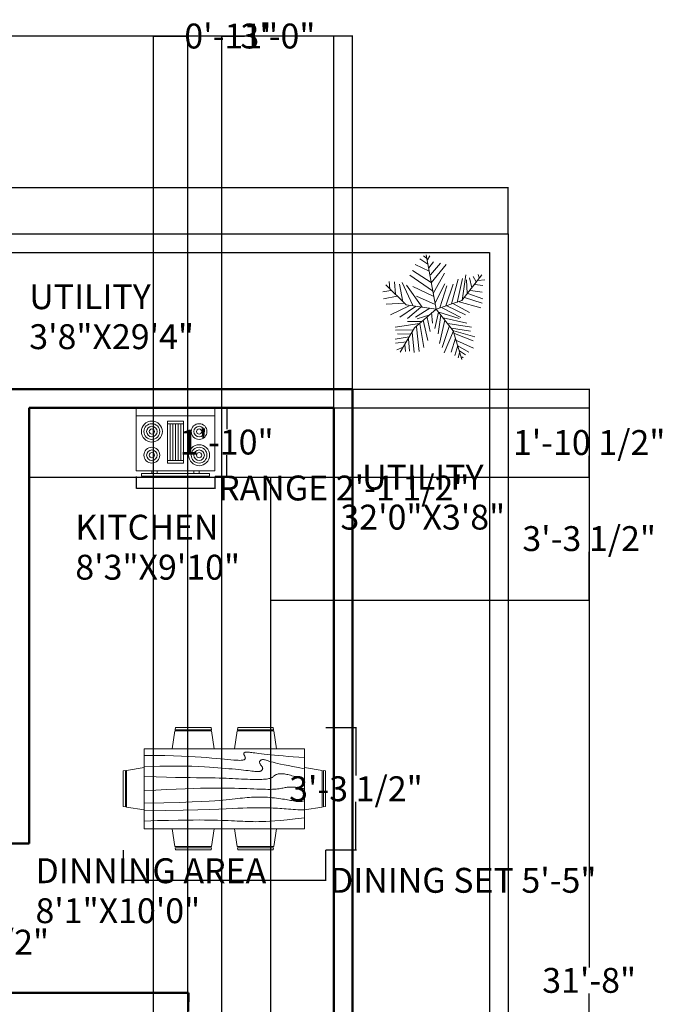
# Model space of a CAD drawing. Units: inches. Extents: x -1912 to -1462, y -785 to -198.
# Tile 3 of 3: x -1668 to -1462, y -515 to -198. Entities that reach past the tile are written whole.
import ezdxf
from ezdxf.enums import TextEntityAlignment as Align

# ---------------------------------------------------------------- set-up
doc = ezdxf.new("R2010")
doc.units = ezdxf.units.IN
doc.header["$MEASUREMENT"] = 0
for name, color, linetype, lineweight in [('A-ANNO-DIMS', 2, 'Continuous', 18), ('A-AREA-IDEN', 7, 'Continuous', 18), ('A-EQPM', 9, 'Continuous', 18), ('A-FLOR-CASE', 9, 'Continuous', 25), ('A-FURN', 8, 'Continuous', 18), ('A-WALL', 7, 'Continuous', 50), ('C-PROP', 8, 'Continuous', 25), ('L-PLNT-TREE', 3, 'Continuous', 13)]:
    doc.layers.add(name, color=color, linetype=linetype, lineweight=lineweight)
doc.styles.get("Standard").update_dxf_attribs({"font": 'arial.ttf'})
doc.dimstyles.get("Standard").update_dxf_attribs({"dimtxt": 8, "dimasz": 0.18, "dimexe": 0.18, "dimexo": 0.0625, "dimgap": 0.09, "dimtad": 0, "dimtih": 1, "dimtoh": 1, "dimzin": 0, "dimdsep": 46, "dimlunit": 3, "dimtxsty": 'Standard', "dimcen": 0.09, "dimadec": 0, "dimazin": 0, "dimtfac": 1, "dimtofl": 0, "dimtmove": 0, "dimatfit": 3, "dimfxl": 1, "dimtolj": 1, "dimtzin": 0, "dimarcsym": 0})

# ---------------------------------------------------------------- blocks, each defined once
blk = doc.blocks.new('Dining Set - 36 x 72 in.')
for p, q in [((-22, 27.5), (-22.1562, 26.50042)), ((-22, 27.5), (-6, 27.5)), ((-5.8437, 26.49966), (-6, 27.5)), ((6, 27.5), (5.8438, 26.50042)), ((6, 27.5), (22, 27.5)), ((22.1563, 26.49966), (22, 27.5)), ((-22.2343, 26.00059), (-23.4847, 17.99762)), ((-22.2304, 26), (-5.7608, 26)), ((-5.8416, 26.5), (-22.1534, 26.5)), ((-4.5152, 17.99762), (-5.7655, 25.99926)), ((5.7657, 26.00059), (4.5153, 17.99762)), ((5.7696, 26), (22.2392, 26)), ((22.1584, 26.5), (5.8466, 26.5)), ((23.4848, 17.99762), (22.2345, 25.99926)), ((36, 18), (-36, 18)), ((-36, 18), (-36, -18)), ((36, -18), (36, 18)), ((-44.0006, 8.23428), (-35.9976, 9.48474)), ((44.0006, 8.23428), (35.9976, 9.48474)), ((-45.5, 8), (-44.5004, 8.15617)), ((-45.5, 8), (-45.5, -8)), ((-44.5, -8.15843), (-44.5, 8.15338)), ((-44, 8.23041), (-44, -8.23915)), ((44, 8.23041), (44, -8.23915)), ((44.5, -8.15843), (44.5, 8.15338)), ((45.5, 8), (44.5005, 8.15617)), ((45.5, 8), (45.5, -8)), ((-44.4997, -8.15631), (-45.5, -8)), ((-35.9976, -9.48476), (-43.9993, -8.2345)), ((35.9976, -9.48476), (43.9993, -8.2345)), ((44.4997, -8.15631), (45.5, -8)), ((-36, -18), (36, -18)), ((-22.2343, -26.0006), (-23.4847, -17.99762)), ((-4.5152, -17.99762), (-5.7655, -25.99928)), ((5.7657, -26.0006), (4.5153, -17.99762)), ((23.4848, -17.99762), (22.2345, -25.99928)), ((-22.2304, -26), (-5.7608, -26)), ((-22, -27.5), (-22.1562, -26.50044)), ((-5.8416, -26.5), (-22.1534, -26.5)), ((-5.8437, -26.49967), (-6, -27.5)), ((5.7696, -26), (22.2392, -26)), ((6, -27.5), (5.8438, -26.50044)), ((22.1584, -26.5), (5.8466, -26.5)), ((22.1563, -26.49967), (22, -27.5)), ((-22, -27.5), (-6, -27.5)), ((6, -27.5), (22, -27.5))]:
    blk.add_line(p, q)
for points in [[(-36, 15), (-31.1772, 14.97754), (-26.8079, 14.91406), (-22.8538, 14.81543), (-19.276, 14.6875), (-16.0362, 14.53613), (-13.0957, 14.36718), (-10.4159, 14.18652), (-7.9583, 14), (-5.6904, 13.81315), (-3.6035, 13.63021), (-1.6954, 13.45508), (0.0365, 13.29166), (1.5945, 13.14388), (2.9811, 13.01562), (4.1988, 12.9108), (5.25, 12.83333), (6.1393, 12.78613), (6.8802, 12.76823), (7.4883, 12.77767), (7.9792, 12.8125), (8.3685, 12.87077), (8.6719, 12.95052), (8.9049, 13.0498), (9.0833, 13.16666), (9.2205, 13.29899), (9.3216, 13.44401), (9.3895, 13.59879), (9.4271, 13.76041), (9.4373, 13.92594), (9.4232, 14.09245), (9.3875, 14.257), (9.3333, 14.41666), (9.2638, 14.56917), (9.1836, 14.71484), (9.0975, 14.85465), (9.0104, 14.98958), (8.9272, 15.1206), (8.8529, 15.2487), (8.7922, 15.37483), (8.75, 15.5), (8.7305, 15.62467), (8.7344, 15.74739), (8.7617, 15.86621), (8.8125, 15.97916), (8.8867, 16.08431), (8.9844, 16.17968), (9.1055, 16.26334), (9.25, 16.33333), (9.4189, 16.38802), (9.6172, 16.42708), (9.8506, 16.45052), (10.125, 16.45833), (10.4463, 16.45052), (10.8203, 16.42708), (11.2529, 16.38802), (11.75, 16.33333), (12.3184, 16.26318), (12.9694, 16.17838), (13.7151, 16.07991), (14.5677, 15.96875), (15.5395, 15.84586), (16.6426, 15.71224), (17.8893, 15.56884), (19.2917, 15.41666), (20.859, 15.25667), (22.5879, 15.08984), (24.4721, 14.91715), (26.5052, 14.73958), (28.6809, 14.5581), (30.9929, 14.3737), (33.4347, 14.18733), (36, 14)], [(-36, 10), (-28.9766, 10.14274), (-23.1725, 10.20442), (-18.4241, 10.19775), (-14.5677, 10.13541), (-11.4399, 10.03011), (-8.877, 9.89453), (-6.7154, 9.74137), (-4.7917, 9.58333), (-2.9698, 9.43082), (-1.2246, 9.28515), (0.4415, 9.14534), (2.026, 9.01041), (3.5266, 8.87939), (4.9408, 8.7513), (6.266, 8.62516), (7.5, 8.5), (8.6411, 8.37549), (9.6914, 8.2539), (10.6538, 8.13818), (11.5312, 8.03125), (12.3267, 7.93603), (13.043, 7.85547), (13.6831, 7.79248), (14.25, 7.75), (14.7471, 7.7303), (15.1797, 7.73307), (15.5537, 7.75732), (15.875, 7.80208), (16.1494, 7.86637), (16.3828, 7.94922), (16.5811, 8.04964), (16.75, 8.16666), (16.8944, 8.29915), (17.0143, 8.44531), (17.1089, 8.60319), (17.1771, 8.77083), (17.218, 8.94629), (17.2305, 9.1276), (17.2137, 9.31282), (17.1667, 9.5), (17.0895, 9.6875), (16.987, 9.875), (16.8649, 10.0625), (16.7292, 10.25), (16.5856, 10.4375), (16.4401, 10.625), (16.2985, 10.8125), (16.1667, 11), (16.05, 11.18733), (15.9518, 11.3737), (15.8752, 11.5581), (15.8229, 11.73958), (15.798, 11.91715), (15.8034, 12.08984), (15.842, 12.25667), (15.9167, 12.41666), (16.0295, 12.56836), (16.1784, 12.70833), (16.3605, 12.83268), (16.5729, 12.9375), (16.8127, 13.01888), (17.0768, 13.07291), (17.3625, 13.0957), (17.6667, 13.08333), (17.9894, 13.03312), (18.3418, 12.94726), (18.7382, 12.82918), (19.1927, 12.68229), (19.7195, 12.51001), (20.3327, 12.31575), (21.0465, 12.10294), (21.875, 11.875), (22.8357, 11.63354), (23.959, 11.37304), (25.2786, 11.08618), (26.8282, 10.76562), (28.6414, 10.40405), (30.752, 9.99414), (33.1936, 9.52856), (36, 9)], [(-36, 5.5), (-30.7157, 5.3348), (-26.069, 5.20963), (-21.9946, 5.11767), (-18.4271, 5.05208), (-15.3009, 5.00602), (-12.5508, 4.97265), (-10.1112, 4.94515), (-7.9167, 4.91666), (-5.909, 4.88167), (-4.0586, 4.83984), (-2.3429, 4.79215), (-0.7396, 4.73958), (0.7739, 4.6831), (2.22, 4.6237), (3.6213, 4.56233), (5, 4.5), (6.373, 4.43782), (7.7344, 4.3776), (9.0723, 4.32129), (10.375, 4.27083), (11.6309, 4.22819), (12.8281, 4.19531), (13.9551, 4.17415), (15, 4.16666), (15.954, 4.17448), (16.819, 4.19791), (17.6001, 4.23698), (18.3021, 4.29166), (18.9299, 4.36198), (19.4883, 4.44791), (19.9823, 4.54948), (20.4167, 4.66666), (20.7969, 4.79899), (21.1302, 4.94401), (21.4245, 5.09879), (21.6875, 5.26041), (21.9271, 5.42594), (22.1511, 5.59245), (22.3672, 5.757), (22.5834, 5.91666), (22.8065, 6.06868), (23.0404, 6.21093), (23.2879, 6.34147), (23.5521, 6.45833), (23.8358, 6.55957), (24.142, 6.64323), (24.4735, 6.70735), (24.8334, 6.75), (25.2235, 6.76969), (25.642, 6.76692), (26.0858, 6.74267), (26.5521, 6.69791), (27.0379, 6.63362), (27.5404, 6.55078), (28.0565, 6.45036), (28.5834, 6.33333), (29.1242, 6.19987), (29.7071, 6.04687), (30.3661, 5.87044), (31.1354, 5.66666), (32.0493, 5.43164), (33.142, 5.16146), (34.4475, 4.85221), (36, 4.5)], [(-36, -1), (-30.7915, -0.6591), (-26.0195, -0.38216), (-21.6519, -0.16284), (-17.6563, 0.00521), (-14.0005, 0.12833), (-10.6523, 0.21289), (-7.5796, 0.26522), (-4.75, 0.29166), (-2.134, 0.29793), (0.2878, 0.28711), (2.5317, 0.26163), (4.6146, 0.22396), (6.5529, 0.17651), (8.3633, 0.12174), (10.0623, 0.06209), (11.6667, 0), (13.1899, -0.06201), (14.6341, -0.1211), (15.9982, -0.17432), (17.2813, -0.21875), (18.4823, -0.25147), (19.6003, -0.26953), (20.6343, -0.27002), (21.5834, -0.25), (22.4481, -0.20768), (23.2357, -0.14584), (23.9549, -0.06836), (24.6146, 0.02083), (25.2235, 0.11784), (25.7904, 0.21875), (26.3241, 0.31966), (26.8334, 0.41666), (27.3265, 0.50618), (27.8099, 0.58593), (28.2894, 0.65397), (28.7709, 0.70833), (29.2601, 0.74707), (29.763, 0.76823), (30.2855, 0.76985), (30.8334, 0.75), (31.4088, 0.70784), (31.9994, 0.64713), (32.589, 0.57275), (33.1615, 0.48958), (33.7008, 0.4025), (34.1908, 0.3164), (34.6153, 0.23616), (34.9584, 0.16666), (35.2099, 0.11165), (35.3848, 0.07031), (35.504, 0.04069), (35.5886, 0.02083), (35.6594, 0.00879), (35.7377, 0.0026), (35.8442, 0.00032), (36, 0)], [(-36, -6.5), (-27.1843, -6.31267), (-20.084, -6.1263), (-14.469, -5.9419), (-10.1094, -5.76042), (-6.7752, -5.58285), (-4.2363, -5.41016), (-2.2629, -5.24333), (-0.625, -5.08334), (0.8708, -4.93099), (2.2715, -4.78646), (3.5872, -4.64974), (4.8281, -4.52084), (6.0046, -4.39974), (7.127, -4.28646), (8.2053, -4.18099), (9.25, -4.08334), (10.2705, -3.99382), (11.2734, -3.91407), (12.2647, -3.84603), (13.25, -3.79167), (14.2354, -3.75293), (15.2266, -3.73177), (16.2295, -3.73015), (17.25, -3.75), (18.2912, -3.79248), (19.3451, -3.85547), (20.4009, -3.93604), (21.4479, -4.03125), (22.4754, -4.13819), (23.4727, -4.25391), (24.4289, -4.37549), (25.3334, -4.5), (26.1785, -4.62492), (26.9694, -4.74935), (27.7145, -4.87281), (28.4219, -4.99479), (29.1, -5.11483), (29.7572, -5.23242), (30.4016, -5.34709), (31.0417, -5.45834), (31.6837, -5.56437), (32.3262, -5.65821), (32.9658, -5.73153), (33.599, -5.77604), (34.2224, -5.78345), (34.8327, -5.74545), (35.4264, -5.65373), (36, -5.5)], [(-36, -10), (-26.4022, -9.81299), (-18.4675, -9.62891), (-11.9839, -9.45069), (-6.7396, -9.28125), (-2.5226, -9.12354), (0.8789, -8.98047), (3.6769, -8.85498), (6.0833, -8.75), (8.2767, -8.66765), (10.3021, -8.60677), (12.1712, -8.56543), (13.8958, -8.54167), (15.4876, -8.53353), (16.9583, -8.53907), (18.3197, -8.55632), (19.5834, -8.58334), (20.7616, -8.61841), (21.8685, -8.66081), (22.9188, -8.71004), (23.9271, -8.76563), (24.9081, -8.82707), (25.8763, -8.89388), (26.8465, -8.96558), (27.8334, -9.04167), (28.8474, -9.12118), (29.8828, -9.20117), (30.93, -9.27824), (31.9792, -9.34896), (33.0205, -9.40991), (34.0443, -9.45768), (35.0407, -9.48885), (36, -9.5)], [(-36, -14.5), (-30.0881, -14.33513), (-25.0332, -14.21224), (-20.7312, -14.12647), (-17.0781, -14.07292), (-13.97, -14.04671), (-11.3027, -14.04297), (-8.9724, -14.05681), (-6.875, -14.08334), (-4.9224, -14.11833), (-3.0905, -14.16016), (-1.3709, -14.20785), (0.2448, -14.26042), (1.7647, -14.3169), (3.1973, -14.3763), (4.5507, -14.43767), (5.8333, -14.5), (7.0554, -14.5621), (8.235, -14.62175), (9.3922, -14.67652), (10.5469, -14.72396), (11.7192, -14.76164), (12.929, -14.78711), (14.1965, -14.79794), (15.5417, -14.79167), (16.9933, -14.76424), (18.6152, -14.70508), (20.4804, -14.60197), (22.6615, -14.44271), (25.2312, -14.21509), (28.2624, -13.9069), (31.8277, -13.50594), (36, -13)]]:
    blk.add_lwpolyline(points)
blk = doc.blocks.new('Range-Oven - 30 in top')
for p, q in [((0, -3), (30, -3)), ((12, -6), (18, -6)), ((13, -20), (13, -6)), ((14, -6), (14, -20)), ((15, -20), (15, -6)), ((16, -6), (16, -20)), ((17, -20), (17, -6)), ((18, -20), (12, -20)), ((6, -24), (6, -25)), ((8, -25), (8, -24)), ((22, -25), (22, -24)), ((24, -24), (24, -25))]:
    blk.add_line(p, q)
for points in [[(0, -24), (0, 0), (30, 0), (30, -24)], [(12, -21), (12, -5), (18, -5), (18, -21)], [(2, -26), (2, -25), (28, -25), (28, -26)]]:
    blk.add_lwpolyline(points, close=True)
for centre, radius in [((6, -9), 4), ((6, -9), 3), ((6, -9), 2), ((24, -9), 3), ((24, -9), 2), ((6, -9), 1), ((24, -9), 1), ((24, -18), 4), ((6, -18), 3), ((6, -18), 2), ((6, -18), 1), ((24, -18), 3), ((24, -18), 2), ((24, -18), 1)]:
    blk.add_circle(centre, radius)
blk = doc.blocks.new('*U11')
for p, q in [((-8.737, 47.138), (-17.069, 52.711)), ((-10.186, 53.64), (-13.084, 55.962)), ((0, 0), (-10.5, 57)), ((-9.099, 51.782), (-6.563, 55.962)), ((-7.288, 39.707), (-21.778, 46.673)), ((-7.65, 43.423), (-2.578, 49.46)), ((-5.839, 35.992), (4.667, 48.067)), ((-5.114, 27.632), (10.463, 46.673)), ((-3.665, 19.273), (-27.574, 35.527)), ((-5.114, 28.097), (-24.676, 40.636)), ((-2.941, 16.486), (8.652, 37.85)), ((16.259, 5.805), (23.142, 31.348)), ((22.055, 7.198), (27.489, 32.277)), ((27, 9), (48, 36)), ((27.127, 9.056), (31.112, 35.992)), ((35.096, 32.741), (37.27, 22.524)), ((38.719, 34.134), (41.979, 28.561)), ((44.153, 36.456), (45.239, 32.741)), ((-31.5, 4.5), (-52.5, 25.5)), ((-48.585, 21.131), (-49.309, 29.026)), ((-43.513, 28.561), (-42.427, 15.558)), ((-38.442, 26.239), (-34.819, 7.663)), ((-35.544, 28.097), (-24.314, 3.947)), ((-14.533, 2.09), (-30.834, 25.31)), ((-24.314, 23.917), (-2.941, 13.7)), ((-1.129, 6.734), (9.014, 26.704)), ((3.942, 1.625), (11.187, 24.381)), ((10.101, 3.483), (17.708, 26.239)), ((31.836, 30.883), (32.561, 16.486)), ((40.53, 25.775), (48.862, 24.846)), ((43.791, 29.954), (51.036, 30.883)), ((-47.498, 19.737), (-55.83, 18.344)), ((-40.615, 13.7), (-55.105, 10.913)), ((-20.691, 13.7), (-1.129, 4.876)), ((29.662, 12.307), (48.137, 6.269)), ((33.285, 16.486), (48.862, 10.913)), ((36.183, 19.737), (48.137, 17.88)), ((-33.37, 6.269), (-52.207, 5.34)), ((-28.299, 3.483), (-47.86, -5.805)), ((-21.416, 3.018), (-38.079, -8.128)), ((0, 0), (-31.5, 4.5)), ((-15.982, 2.09), (-30.11, -9.521)), ((0, 0), (-22.5, -19.5)), ((-6.563, 1.161), (-21.416, -8.128)), ((0, 0), (27, 9)), ((0, 0), (18, -22.5)), ((6.478, 1.625), (26.04, -8.592)), ((11.187, 3.483), (30.749, -5.805)), ((18.07, 5.805), (35.096, -3.483)), ((24.229, 7.663), (46.688, 1.625)), ((-6.563, -5.805), (-19.967, -9.985)), ((-9.461, -8.592), (-6.201, -23.453)), ((-4.752, -3.483), (-3.665, -14.629)), ((2.493, -3.019), (-1.491, -20.202)), ((1.769, -2.555), (24.229, -9.521)), ((5.029, -6.27), (2.131, -25.775)), ((7.565, -9.056), (32.198, -14.629)), ((-17.431, -15.094), (-42.789, -18.809)), ((-22.5, -19.5), (-37.5, -45)), ((-15.257, -12.772), (-30.11, -12.772)), ((-20.691, -18.345), (-17.793, -44.352)), ((-17.069, -15.094), (-12.721, -40.172)), ((-13.446, -11.378), (-8.737, -32.741)), ((9.014, -11.378), (3.58, -35.992)), ((14.085, -16.951), (6.478, -40.172)), ((12.274, -15.094), (36.907, -18.809)), ((16.259, -19.738), (36.183, -22.989)), ((-28.299, -29.026), (-42.789, -31.348)), ((-24.314, -21.596), (-42.427, -22.06)), ((-26.849, -26.24), (-40.253, -25.775)), ((-29.023, -30.884), (-27.936, -43.887)), ((-25.038, -23.918), (-22.865, -45.281)), ((18.07, -22.524), (8.289, -45.745)), ((20.244, -30.419), (15.897, -44.816)), ((18, -22.5), (27, -52.5)), ((18.433, -22.524), (40.53, -29.026)), ((19.157, -25.311), (38.719, -33.206)), ((-30.834, -34.135), (-42.427, -35.528)), ((-34.457, -39.708), (-40.978, -42.494)), ((-32.646, -36.921), (-31.921, -44.352)), ((22.78, -37.85), (19.519, -48.532)), ((21.331, -32.741), (39.081, -40.636)), ((22.78, -38.314), (34.372, -44.816)), ((24.591, -45.745), (23.142, -50.854)), ((24.591, -43.423), (30.749, -47.603)), ((26.764, -49.925), (28.213, -50.854))]:
    blk.add_line(p, q)
blk = doc.blocks.new('*D12')
at = {"layer": 'A-ANNO-DIMS', "color": 0, "lineweight": -2, "transparency": 16777216}
for p, q in [((-1871.08, -267.18), (-1871.08, -252.32)), ((-1870.9, -252.5), (-1697.95, -252.5)), ((-1511.26, -252.5), (-1684.2, -252.5)), ((-1511.08, -267.18), (-1511.08, -252.32))]:
    blk.add_line(p, q, dxfattribs=at)
at = {"layer": 'A-ANNO-DIMS', "color": 0, "transparency": 16777216}
for points in [[(-1870.9, -252.47), (-1870.9, -252.53), (-1871.08, -252.5)], [(-1511.26, -252.47), (-1511.26, -252.53), (-1511.08, -252.5)]]:
    blk.add_solid(points, dxfattribs=at)
at = {"layer": 'Defpoints', "color": 0, "transparency": 16777216}
for p in [(-1511.08, -252.5), (-1871.08, -267.24), (-1511.08, -267.24)]:
    blk.add_point(p, dxfattribs=at)
at = {"layer": 'A-ANNO-DIMS', "color": 0, "transparency": 16777216, "insert": (-1691.08, -252.5), "char_height": 8, "attachment_point": 5}
blk.add_mtext("\\A1;30'", dxfattribs=at)
blk = doc.blocks.new('*D17')
at = {"layer": 'A-ANNO-DIMS', "color": 0, "lineweight": -2, "transparency": 16777216}
for p, q in [((-1742.16, -491.83), (-1742.16, -495.14)), ((-1720.86, -491.83), (-1720.86, -495.14)), ((-1741.98, -494.96), (-1721.04, -494.96)), ((-1720.86, -494.96), (-1720.68, -494.96))]:
    blk.add_line(p, q, dxfattribs=at)
at = {"layer": 'A-ANNO-DIMS', "color": 0, "transparency": 16777216}
for points in [[(-1741.98, -494.93), (-1741.98, -494.99), (-1742.16, -494.96)], [(-1721.04, -494.93), (-1721.04, -494.99), (-1720.86, -494.96)]]:
    blk.add_solid(points, dxfattribs=at)
at = {"layer": 'Defpoints', "color": 0, "transparency": 16777216}
for p in [(-1742.16, -491.77), (-1720.86, -491.77), (-1720.86, -494.96)]:
    blk.add_point(p, dxfattribs=at)
at = {"layer": 'A-ANNO-DIMS', "color": 0, "transparency": 16777216, "insert": (-1689.61, -494.96), "char_height": 8, "attachment_point": 5}
blk.add_mtext('\\A1;WC 1\'-9 1/2"', dxfattribs=at)
blk = doc.blocks.new('*D27')
at = {"layer": 'A-ANNO-DIMS', "color": 0, "lineweight": -2, "transparency": 16777216}
for p, q in [((-1634.83, -465.38), (-1634.83, -475.26)), ((-1569.75, -465.38), (-1569.75, -475.26)), ((-1634.65, -475.08), (-1569.93, -475.08)), ((-1569.75, -475.08), (-1569.57, -475.08))]:
    blk.add_line(p, q, dxfattribs=at)
at = {"layer": 'A-ANNO-DIMS', "color": 0, "transparency": 16777216}
for points in [[(-1634.65, -475.05), (-1634.65, -475.11), (-1634.83, -475.08)], [(-1569.93, -475.05), (-1569.93, -475.11), (-1569.75, -475.08)]]:
    blk.add_solid(points, dxfattribs=at)
at = {"layer": 'Defpoints', "color": 0, "transparency": 16777216}
for p in [(-1634.83, -465.31), (-1569.75, -465.31), (-1569.75, -475.08)]:
    blk.add_point(p, dxfattribs=at)
at = {"layer": 'A-ANNO-DIMS', "color": 0, "transparency": 16777216, "insert": (-1525.52, -475.08), "char_height": 8, "attachment_point": 5}
blk.add_mtext('\\A1;DINING SET 5\'-5"', dxfattribs=at)
blk = doc.blocks.new('*D28')
at = {"layer": 'A-ANNO-DIMS', "color": 0, "lineweight": -2, "transparency": 16777216}
for p, q in [((-1569.69, -425.98), (-1559.81, -425.98)), ((-1559.99, -426.16), (-1559.99, -441.42)), ((-1559.99, -465.13), (-1559.99, -449.88)), ((-1569.69, -465.31), (-1559.81, -465.31))]:
    blk.add_line(p, q, dxfattribs=at)
at = {"layer": 'A-ANNO-DIMS', "color": 0, "transparency": 16777216}
for points in [[(-1560.02, -426.16), (-1559.96, -426.16), (-1559.99, -425.98)], [(-1560.02, -465.13), (-1559.96, -465.13), (-1559.99, -465.31)]]:
    blk.add_solid(points, dxfattribs=at)
at = {"layer": 'Defpoints', "color": 0, "transparency": 16777216}
for p in [(-1569.75, -425.98), (-1559.99, -425.98), (-1569.75, -465.31)]:
    blk.add_point(p, dxfattribs=at)
at = {"layer": 'A-ANNO-DIMS', "color": 0, "transparency": 16777216, "insert": (-1559.99, -445.65), "char_height": 8, "attachment_point": 5}
blk.add_mtext('\\A1;3\'-3 1/2"', dxfattribs=at)
blk = doc.blocks.new('*D31')
at = {"layer": 'A-ANNO-DIMS', "color": 0, "lineweight": -2, "transparency": 16777216}
for p, q in [((-1630.66, -345.25), (-1630.66, -349.17)), ((-1605.34, -345.25), (-1605.34, -349.17)), ((-1630.48, -348.99), (-1605.52, -348.99)), ((-1605.34, -348.99), (-1605.16, -348.99))]:
    blk.add_line(p, q, dxfattribs=at)
at = {"layer": 'A-ANNO-DIMS', "color": 0, "transparency": 16777216}
for points in [[(-1630.48, -348.96), (-1630.48, -349.02), (-1630.66, -348.99)], [(-1605.52, -348.96), (-1605.52, -349.02), (-1605.34, -348.99)]]:
    blk.add_solid(points, dxfattribs=at)
at = {"layer": 'Defpoints', "color": 0, "transparency": 16777216}
for p in [(-1630.66, -345.19), (-1605.34, -345.19), (-1605.34, -348.99)]:
    blk.add_point(p, dxfattribs=at)
at = {"layer": 'A-ANNO-DIMS', "color": 0, "transparency": 16777216, "insert": (-1563.9, -348.99), "char_height": 8, "attachment_point": 5}
blk.add_mtext('\\A1;RANGE 2\'-1 1/2"', dxfattribs=at)
blk = doc.blocks.new('*D32')
at = {"layer": 'A-ANNO-DIMS', "color": 0, "lineweight": -2, "transparency": 16777216}
for p, q in [((-1605.28, -323.25), (-1601.36, -323.25)), ((-1601.54, -323.43), (-1601.54, -330.04)), ((-1601.54, -345.01), (-1601.54, -338.39)), ((-1605.28, -345.19), (-1601.36, -345.19))]:
    blk.add_line(p, q, dxfattribs=at)
at = {"layer": 'A-ANNO-DIMS', "color": 0, "transparency": 16777216}
for points in [[(-1601.57, -323.43), (-1601.51, -323.43), (-1601.54, -323.25)], [(-1601.57, -345.01), (-1601.51, -345.01), (-1601.54, -345.19)]]:
    blk.add_solid(points, dxfattribs=at)
at = {"layer": 'Defpoints', "color": 0, "transparency": 16777216}
for p in [(-1605.34, -323.25), (-1601.54, -323.25), (-1605.34, -345.19)]:
    blk.add_point(p, dxfattribs=at)
at = {"layer": 'A-ANNO-DIMS', "color": 0, "transparency": 16777216, "insert": (-1601.54, -334.22), "char_height": 8, "attachment_point": 5}
blk.add_mtext('\\A1;1\'-10"', dxfattribs=at)
blk = doc.blocks.new('*D33')
at = {"layer": 'A-ANNO-DIMS', "color": 0, "lineweight": -2, "transparency": 16777216}
for p, q in [((-1821.08, -317.18), (-1821.08, -203.54)), ((-1820.9, -203.72), (-1704.98, -203.72)), ((-1561.26, -203.72), (-1677.18, -203.72)), ((-1561.08, -317.18), (-1561.08, -203.54))]:
    blk.add_line(p, q, dxfattribs=at)
at = {"layer": 'A-ANNO-DIMS', "color": 0, "transparency": 16777216}
for points in [[(-1820.9, -203.69), (-1820.9, -203.75), (-1821.08, -203.72)], [(-1561.26, -203.69), (-1561.26, -203.75), (-1561.08, -203.72)]]:
    blk.add_solid(points, dxfattribs=at)
at = {"layer": 'Defpoints', "color": 0, "transparency": 16777216}
for p in [(-1561.08, -203.72), (-1821.08, -317.24), (-1561.08, -317.24)]:
    blk.add_point(p, dxfattribs=at)
at = {"layer": 'A-ANNO-DIMS', "color": 0, "transparency": 16777216, "insert": (-1691.08, -203.72), "char_height": 8, "attachment_point": 5}
blk.add_mtext('\\A1;21\'-8"', dxfattribs=at)
blk = doc.blocks.new('*D34')
at = {"layer": 'A-ANNO-DIMS', "color": 0, "lineweight": -2, "transparency": 16777216}
for p, q in [((-1561.02, -317.24), (-1484.85, -317.24)), ((-1485.03, -317.42), (-1485.03, -503.06)), ((-1485.03, -697.06), (-1485.03, -511.42)), ((-1561.02, -697.24), (-1484.85, -697.24))]:
    blk.add_line(p, q, dxfattribs=at)
at = {"layer": 'A-ANNO-DIMS', "color": 0, "transparency": 16777216}
for points in [[(-1485.06, -317.42), (-1485, -317.42), (-1485.03, -317.24)], [(-1485.06, -697.06), (-1485, -697.06), (-1485.03, -697.24)]]:
    blk.add_solid(points, dxfattribs=at)
at = {"layer": 'Defpoints', "color": 0, "transparency": 16777216}
for p in [(-1561.08, -317.24), (-1561.08, -697.24), (-1485.03, -697.24)]:
    blk.add_point(p, dxfattribs=at)
at = {"layer": 'A-ANNO-DIMS', "color": 0, "transparency": 16777216, "insert": (-1485.03, -507.24), "char_height": 8, "attachment_point": 5}
blk.add_mtext('\\A1;31\'-8"', dxfattribs=at)
blk = doc.blocks.new('*D38')
at = {"layer": 'A-ANNO-DIMS', "color": 0, "lineweight": -2, "transparency": 16777216}
for p, q in [((-1603.08, -578.18), (-1603.08, -203.54)), ((-1602.9, -203.72), (-1595.8, -203.72)), ((-1567.26, -203.72), (-1574.36, -203.72)), ((-1567.08, -578.18), (-1567.08, -203.54))]:
    blk.add_line(p, q, dxfattribs=at)
at = {"layer": 'A-ANNO-DIMS', "color": 0, "transparency": 16777216}
for points in [[(-1602.9, -203.69), (-1602.9, -203.75), (-1603.08, -203.72)], [(-1567.26, -203.69), (-1567.26, -203.75), (-1567.08, -203.72)]]:
    blk.add_solid(points, dxfattribs=at)
at = {"layer": 'Defpoints', "color": 0, "transparency": 16777216}
for p in [(-1567.08, -203.72), (-1603.08, -578.24), (-1567.08, -578.24)]:
    blk.add_point(p, dxfattribs=at)
at = {"layer": 'A-ANNO-DIMS', "color": 0, "transparency": 16777216, "insert": (-1585.08, -203.72), "char_height": 8, "attachment_point": 5}
blk.add_mtext('\\A1;3\'-0"', dxfattribs=at)
blk = doc.blocks.new('*D39')
at = {"layer": 'A-ANNO-DIMS', "color": 0, "lineweight": -2, "transparency": 16777216}
for p, q in [((-1625.08, -655.18), (-1625.08, -203.54)), ((-1624.9, -203.72), (-1614.26, -203.72)), ((-1614.08, -655.18), (-1614.08, -203.54)), ((-1614.08, -203.72), (-1613.9, -203.72))]:
    blk.add_line(p, q, dxfattribs=at)
at = {"layer": 'A-ANNO-DIMS', "color": 0, "transparency": 16777216}
for points in [[(-1624.9, -203.69), (-1624.9, -203.75), (-1625.08, -203.72)], [(-1614.26, -203.69), (-1614.26, -203.75), (-1614.08, -203.72)]]:
    blk.add_solid(points, dxfattribs=at)
at = {"layer": 'Defpoints', "color": 0, "transparency": 16777216}
for p in [(-1614.08, -203.72), (-1625.08, -655.24), (-1614.08, -655.24)]:
    blk.add_point(p, dxfattribs=at)
at = {"layer": 'A-ANNO-DIMS', "color": 0, "transparency": 16777216, "insert": (-1600.07, -203.72), "char_height": 8, "attachment_point": 5}
blk.add_mtext('\\A1;0\'-11"', dxfattribs=at)
blk = doc.blocks.new('*D41')
at = {"layer": 'A-ANNO-DIMS', "color": 0, "lineweight": -2, "transparency": 16777216}
for p, q in [((-1665.02, -323.24), (-1484.85, -323.24)), ((-1485.03, -323.42), (-1485.03, -330.14)), ((-1485.03, -345.32), (-1485.03, -338.6)), ((-1665.02, -345.5), (-1484.85, -345.5))]:
    blk.add_line(p, q, dxfattribs=at)
at = {"layer": 'A-ANNO-DIMS', "color": 0, "transparency": 16777216}
for points in [[(-1485.06, -323.42), (-1485, -323.42), (-1485.03, -323.24)], [(-1485.06, -345.32), (-1485, -345.32), (-1485.03, -345.5)]]:
    blk.add_solid(points, dxfattribs=at)
at = {"layer": 'Defpoints', "color": 0, "transparency": 16777216}
for p in [(-1665.08, -323.24), (-1665.08, -345.5), (-1485.03, -345.5)]:
    blk.add_point(p, dxfattribs=at)
at = {"layer": 'A-ANNO-DIMS', "color": 0, "transparency": 16777216, "insert": (-1485.03, -334.37), "char_height": 8, "attachment_point": 5}
blk.add_mtext('\\A1;1\'-10 1/2"', dxfattribs=at)
blk = doc.blocks.new('*D42')
at = {"layer": 'A-ANNO-DIMS', "color": 0, "lineweight": -2, "transparency": 16777216}
for p, q in [((-1587.5, -385.06), (-1587.5, -773.47)), ((-1567.08, -385.06), (-1567.08, -773.47)), ((-1587.32, -773.29), (-1567.26, -773.29)), ((-1567.08, -773.29), (-1566.9, -773.29))]:
    blk.add_line(p, q, dxfattribs=at)
at = {"layer": 'A-ANNO-DIMS', "color": 0, "transparency": 16777216}
for points in [[(-1587.32, -773.26), (-1587.32, -773.32), (-1587.5, -773.29)], [(-1567.26, -773.26), (-1567.26, -773.32), (-1567.08, -773.29)]]:
    blk.add_solid(points, dxfattribs=at)
at = {"layer": 'Defpoints', "color": 0, "transparency": 16777216}
for p in [(-1587.5, -385), (-1567.08, -385), (-1567.08, -773.29)]:
    blk.add_point(p, dxfattribs=at)
at = {"layer": 'A-ANNO-DIMS', "color": 0, "transparency": 16777216, "insert": (-1547.23, -773.29), "char_height": 8, "attachment_point": 5}
blk.add_mtext('\\A1;1\'-8 1/2"', dxfattribs=at)
blk = doc.blocks.new('*D43')
at = {"layer": 'A-ANNO-DIMS', "color": 0, "lineweight": -2, "transparency": 16777216}
for p, q in [((-1587.44, -345.5), (-1484.85, -345.5)), ((-1485.03, -345.68), (-1485.03, -361.02)), ((-1485.03, -384.82), (-1485.03, -369.48)), ((-1587.44, -385), (-1484.85, -385))]:
    blk.add_line(p, q, dxfattribs=at)
at = {"layer": 'A-ANNO-DIMS', "color": 0, "transparency": 16777216}
for points in [[(-1485.06, -345.68), (-1485, -345.68), (-1485.03, -345.5)], [(-1485.06, -384.82), (-1485, -384.82), (-1485.03, -385)]]:
    blk.add_solid(points, dxfattribs=at)
at = {"layer": 'Defpoints', "color": 0, "transparency": 16777216}
for p in [(-1587.5, -345.5), (-1485.03, -345.5), (-1587.5, -385)]:
    blk.add_point(p, dxfattribs=at)
at = {"layer": 'A-ANNO-DIMS', "color": 0, "transparency": 16777216, "insert": (-1485.03, -365.25), "char_height": 8, "attachment_point": 5}
blk.add_mtext('\\A1;3\'-3 1/2"', dxfattribs=at)

msp = doc.modelspace()

# ---------------------------------------------------------------- linework, layer by layer
at = {"layer": 'A-FLOR-CASE'}
for p, q in [((-1665.078, -345.5), (-1665.078, -345.5)), ((-1665.078, -345.5), (-1587.5, -345.5)), ((-1587.5, -345.5), (-1587.5, -385)), ((-1587.5, -385), (-1567.078, -385))]:
    msp.add_line(p, q, dxfattribs=at)
at = {"layer": 'A-WALL'}
for p, q in [((-1821.078, -317.241), (-1561.078, -317.241)), ((-1561.078, -317.241), (-1561.078, -697.241)), ((-1665.078, -463.241), (-1665.078, -323.241)), ((-1665.078, -323.241), (-1567.078, -323.241)), ((-1567.078, -323.241), (-1567.078, -691.241)), ((-1675.078, -463.241), (-1665.078, -463.241)), ((-1715.078, -511.241), (-1613.799, -511.241)), ((-1613.924, -517.241), (-1613.799, -511.241))]:
    msp.add_line(p, q, dxfattribs=at)
at = {"layer": 'C-PROP'}
for p, q in [((-1865.078, -273.241), (-1517.078, -273.241)), ((-1517.078, -273.241), (-1517.078, -741.241))]:
    msp.add_line(p, q, dxfattribs=at)
msp.add_lwpolyline([(-1511.078, -747.241), (-1871.078, -747.241), (-1871.078, -267.241), (-1511.078, -267.241)], close=True, dxfattribs=at)

# ---------------------------------------------------------------- block references
at = {"layer": 'A-EQPM', "xscale": 0.8439325934114812, "yscale": 0.8439325934114812, "zscale": 0.8439325934114812}
msp.add_blockref('Range-Oven - 30 in top', (-1630.659, -323.246), dxfattribs=at)
at = {"layer": 'A-FURN', "xscale": 0.7151562624928854, "yscale": 0.7151562624928854, "zscale": 0.7151562624928854}
msp.add_blockref('Dining Set - 36 x 72 in.', (-1602.294, -445.648), dxfattribs=at)
at = {"layer": 'L-PLNT-TREE', "xscale": 0.307023879819639, "yscale": 0.307023879819639, "zscale": 0.307023879819639}
msp.add_blockref('*U11', (-1534.229, -291.531), dxfattribs=at)

# ---------------------------------------------------------------- texts
at = {"layer": 'A-AREA-IDEN'}
for s, p in [('UTILITY', (-1665, -291.5)), ('3\'8"X29\'4"', (-1665, -304.351)), ('KITCHEN', (-1650.201, -365.592)), ('8\'3"X9\'10"', (-1650.201, -378.443)), ('DINNING AREA', (-1663, -476)), ('8\'1"X10\'0"', (-1663, -488.851))]:
    msp.add_text(s, height=8, dxfattribs=at).set_placement(p)
for s, p in [('UTILITY', (-1538.5, -349.5)), ('32\'0"X3\'8"', (-1538.5, -362.351))]:
    msp.add_text(s, height=8, dxfattribs=at).set_placement(p, align=Align.CENTER)

# ---------------------------------------------------------------- dimensions: what is measured, and where the dimension line sits
at = {"layer": 'A-ANNO-DIMS'}
for base, p1, p2, override, picture, middle in [((-1561.078, -203.718), (-1821.078, -317.241), (-1561.078, -317.241), {"dimdec": 1, "dimlfac": 1, "dimrnd": 0, "dimzin": 1, "dimdsep": 46, "dimlunit": 4, "dimfrac": 2}, '*D33', (-1691.078, -203.718)), ((-1614.078, -203.718), (-1625.078, -655.241), (-1614.078, -655.241), {"dimdec": 1, "dimlfac": 1, "dimrnd": 0, "dimzin": 1, "dimdsep": 46, "dimlunit": 4, "dimfrac": 2}, '*D39', (-1600.068, -203.718)), ((-1567.078, -203.718), (-1603.078, -578.241), (-1567.078, -578.241), {"dimdec": 1, "dimlfac": 1, "dimrnd": 0, "dimzin": 1, "dimdsep": 46, "dimlunit": 4, "dimfrac": 2}, '*D38', (-1585.078, -203.718)), ((-1511.078, -252.5), (-1871.078, -267.241), (-1511.078, -267.241), {"dimclrd": 0, "dimclre": 0, "dimclrt": 0}, '*D12', (-1691.078, -252.5)), ((-1567.078, -773.291), (-1587.5, -385), (-1567.078, -385), {"dimdec": 1, "dimlfac": 1, "dimrnd": 0, "dimzin": 1, "dimdsep": 46, "dimlunit": 4, "dimfrac": 2}, '*D42', (-1547.231, -773.291))]:
    dim = msp.add_linear_dim(base=base, p1=p1, p2=p2, dimstyle='Standard', override=override, dxfattribs=at)
    dim.commit()
    dim.dimension.update_dxf_attribs({"geometry": picture, "text_midpoint": middle})
for base, p1, p2, picture, middle in [((-1485.028, -697.241), (-1561.078, -317.241), (-1561.078, -697.241), '*D34', (-1485.028, -507.241)), ((-1485.028, -345.5), (-1665.078, -323.241), (-1665.078, -345.5), '*D41', (-1485.028, -334.37)), ((-1601.543, -323.246), (-1605.341, -345.188), (-1605.341, -323.246), '*D32', (-1601.543, -334.217)), ((-1485.028, -345.5), (-1587.5, -385), (-1587.5, -345.5), '*D43', (-1485.028, -365.25)), ((-1559.992, -425.981), (-1569.754, -465.315), (-1569.754, -425.981), '*D28', (-1559.992, -445.648))]:
    dim = msp.add_linear_dim(base=base, p1=p1, p2=p2, angle=90, dimstyle='Standard', override={"dimdec": 1, "dimlfac": 1, "dimrnd": 0, "dimzin": 1, "dimdsep": 46, "dimlunit": 4, "dimfrac": 2}, dxfattribs=at)
    dim.commit()
    dim.dimension.update_dxf_attribs({"geometry": picture, "text_midpoint": middle})
for base, p1, p2, text, picture, middle in [((-1605.341, -348.986), (-1630.659, -345.188), (-1605.341, -345.188), 'RANGE <>', '*D31', (-1563.9, -348.986)), ((-1569.754, -475.076), (-1634.833, -465.315), (-1569.754, -465.315), 'DINING SET <>', '*D27', (-1525.52, -475.076)), ((-1720.858, -494.963), (-1742.159, -491.768), (-1720.858, -491.768), 'WC <>', '*D17', (-1689.609, -494.963))]:
    dim = msp.add_linear_dim(base=base, p1=p1, p2=p2, text=text, dimstyle='Standard', override={"dimdec": 1, "dimlfac": 1, "dimrnd": 0, "dimzin": 1, "dimdsep": 46, "dimlunit": 4, "dimfrac": 2}, dxfattribs=at)
    dim.commit()
    dim.dimension.update_dxf_attribs({"geometry": picture, "text_midpoint": middle})

doc.saveas('drawing.dxf')
